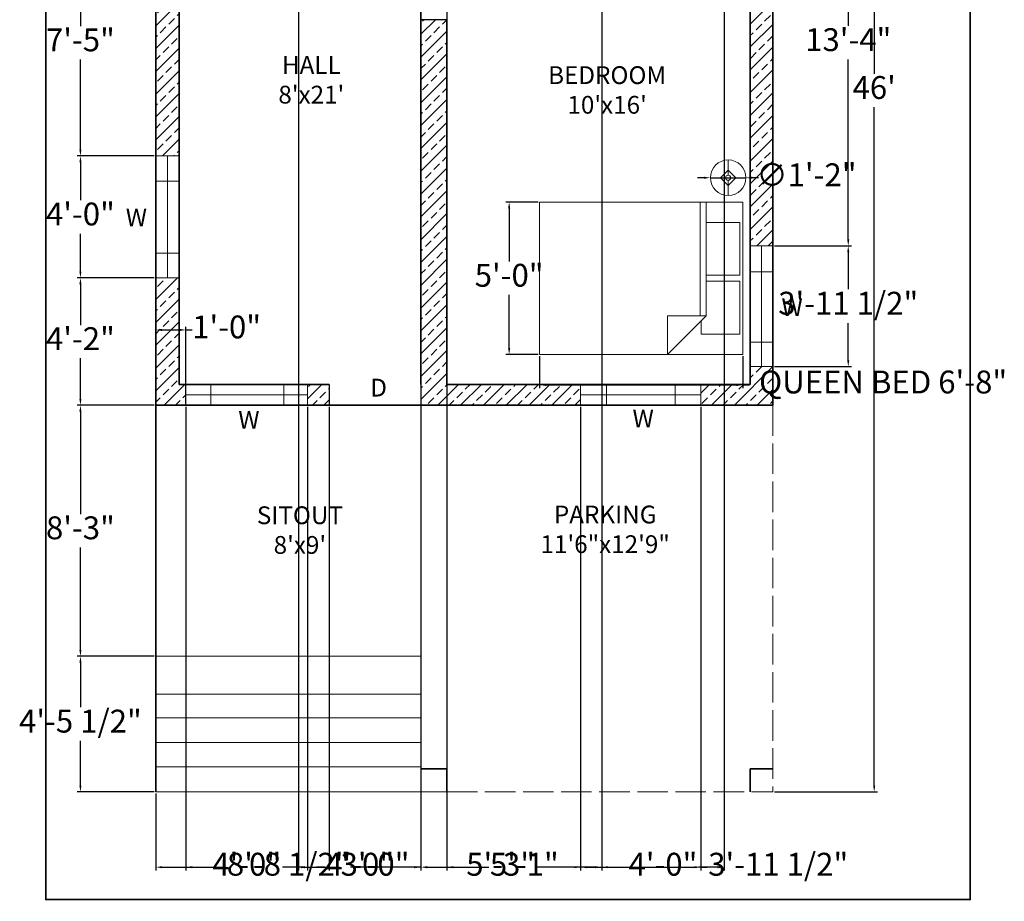
# Model space of a CAD drawing. Units: inches. Extents: x 3686 to 4476, y 4404 to 5066.
# Tile 1 of 2: x 3689 to 4077, y 4404 to 4751. Entities that reach past the tile are written whole.
import ezdxf

# ---------------------------------------------------------------- set-up
doc = ezdxf.new("R2010")
doc.units = ezdxf.units.IN
doc.linetypes.add('ACAD_ISO02W100', pattern=[15, 12, -3])
for name, color, linetype, lineweight in [('A-ANNO-DIMS', 3, 'Continuous', 18), ('A-ANNO-TEXT', 7, 'Continuous', 18), ('A-ANNO-TTLB', 7, 'Continuous', 35), ('A-AREA-IDEN', 7, 'Continuous', 25), ('A-COLS', 7, 'Continuous', 35), ('A-DOOR', 3, 'Continuous', 25), ('A-FLOR-PRKG', 8, 'ACAD_ISO02W100', 18), ('A-FLOR-STRS', 7, 'Continuous', 18), ('A-FURN', 9, 'Continuous', 18), ('A-GLAZ', 4, 'Continuous', 18), ('A-WALL', 7, 'Continuous', 35), ('A-WALL-PATT', 8, 'Continuous', 13)]:
    doc.layers.add(name, color=color, linetype=linetype, lineweight=lineweight)
doc.styles.get("Standard").update_dxf_attribs({"font": 'arial.ttf'})
doc.dimstyles.new('ISO-25', dxfattribs={"dimtxt": 9, "dimasz": 2.5, "dimexe": 1.25, "dimexo": 0.625, "dimgap": 2, "dimtad": 0, "dimtih": 1, "dimtoh": 1, "dimdec": 1, "dimlunit": 4, "dimtxsty": 'Standard', "dimcen": 2.5, "dimadec": 0, "dimazin": 0, "dimtfac": 0.5, "dimtdec": 1, "dimtmove": 0, "dimatfit": 3, "dimfxl": 1, "dimarcsym": 0})

# ---------------------------------------------------------------- blocks, each defined once
blk = doc.blocks.new('*D2')
at = {"layer": 'A-ANNO-DIMS', "color": 0, "lineweight": -2, "transparency": 16777216}
for p, q in [((3986.64, 4999.31), (4027.13, 4999.31)), ((4025.88, 4996.81), (4025.88, 4729.91)), ((4025.88, 4449.81), (4025.88, 4716.72)), ((3986.64, 4447.31), (4027.13, 4447.31))]:
    blk.add_line(p, q, dxfattribs=at)
at = {"layer": 'A-ANNO-DIMS', "color": 0, "transparency": 16777216}
for points in [[(4025.46, 4996.81), (4026.3, 4996.81), (4025.88, 4999.31)], [(4025.46, 4449.81), (4026.3, 4449.81), (4025.88, 4447.31)]]:
    blk.add_solid(points, dxfattribs=at)
at = {"layer": 'Defpoints', "color": 0, "transparency": 16777216}
for p in [(3986.02, 4999.31), (3986.02, 4447.31), (4025.88, 4447.31)]:
    blk.add_point(p, dxfattribs=at)
at = {"layer": 'A-ANNO-DIMS', "color": 0, "transparency": 16777216, "insert": (4025.88, 4723.31), "char_height": 9, "attachment_point": 5}
blk.add_mtext("46'", dxfattribs=at)
blk = doc.blocks.new('Bed - Queen')
for p, q in [((0, -80.00003), (0, 0)), ((0, 0), (59.99999, 0)), ((59.99999, 0), (59.99999, -80.00003)), ((7.99999, -1.2), (28.79998, -1.2)), ((7.99999, -14.4), (7.99999, -1.2)), ((28.79998, -1.2), (28.79998, -14.4)), ((31.19999, -1.2), (51.99999, -1.2)), ((31.19999, -14.4), (31.19999, -1.2)), ((51.99999, -1.2), (51.99999, -16.4)), ((0, -14.4), (44.8, -14.4)), ((59.99999, -29.6), (44.8, -14.4)), ((44.8, -14.4), (44.8, -29.6)), ((44.8, -16.8), (0, -16.8)), ((51.99999, -16.4), (46.79936, -16.4)), ((44.8, -29.6), (59.99999, -29.6)), ((59.99999, -80.00003), (0, -80.00003))]:
    blk.add_line(p, q)
blk = doc.blocks.new('Lamp - Table')
for p, q in [((0, 7), (0, 1)), ((-1, 0), (-7, 0)), ((0, 3), (-3, 0)), ((-3, 0), (0, -3)), ((3, 0), (0, 3)), ((0, -3), (3, 0)), ((1, 0), (7, 0)), ((0, -1), (0, -7))]:
    blk.add_line(p, q)
for radius in [7, 1]:
    blk.add_circle((0, 0), radius)
blk = doc.blocks.new('*D8')
at = {"layer": 'A-ANNO-DIMS', "color": 0, "lineweight": -2, "transparency": 16777216}
for p, q in [((3894.16, 4618.81), (3894.16, 4606.18)), ((3974.16, 4618.81), (3974.16, 4606.18)), ((3896.66, 4607.43), (3971.66, 4607.43)), ((3974.16, 4607.43), (3976.66, 4607.43))]:
    blk.add_line(p, q, dxfattribs=at)
at = {"layer": 'A-ANNO-DIMS', "color": 0, "transparency": 16777216}
for points in [[(3896.66, 4607.85), (3896.66, 4607.02), (3894.16, 4607.43)], [(3971.66, 4607.85), (3971.66, 4607.02), (3974.16, 4607.43)]]:
    blk.add_solid(points, dxfattribs=at)
at = {"layer": 'Defpoints', "color": 0, "transparency": 16777216}
for p in [(3894.16, 4619.43), (3974.16, 4619.43), (3974.16, 4607.43)]:
    blk.add_point(p, dxfattribs=at)
at = {"layer": 'A-ANNO-DIMS', "color": 0, "transparency": 16777216, "insert": (4029.39, 4607.43), "char_height": 9, "attachment_point": 5}
blk.add_mtext('QUEEN BED 6\'-8"', dxfattribs=at)
blk = doc.blocks.new('*D9')
at = {"layer": 'A-ANNO-DIMS', "color": 0, "lineweight": -2, "transparency": 16777216}
for p, q in [((3893.54, 4679.43), (3880.91, 4679.43)), ((3882.16, 4676.93), (3882.16, 4656.03)), ((3882.16, 4621.93), (3882.16, 4642.84)), ((3893.54, 4619.43), (3880.91, 4619.43))]:
    blk.add_line(p, q, dxfattribs=at)
at = {"layer": 'A-ANNO-DIMS', "color": 0, "transparency": 16777216}
for points in [[(3881.75, 4676.93), (3882.58, 4676.93), (3882.16, 4679.43)], [(3881.75, 4621.93), (3882.58, 4621.93), (3882.16, 4619.43)]]:
    blk.add_solid(points, dxfattribs=at)
at = {"layer": 'Defpoints', "color": 0, "transparency": 16777216}
for p in [(3894.16, 4679.43), (3882.16, 4619.43), (3894.16, 4619.43)]:
    blk.add_point(p, dxfattribs=at)
at = {"layer": 'A-ANNO-DIMS', "color": 0, "transparency": 16777216, "insert": (3882.16, 4649.43), "char_height": 9, "attachment_point": 5}
blk.add_mtext('5\'-0"', dxfattribs=at)
blk = doc.blocks.new('*D10')
at = {"layer": 'A-ANNO-DIMS', "color": 0, "lineweight": -2, "transparency": 16777216}
for p, q in [((3742.39, 4599.44), (3712.12, 4599.44)), ((3713.37, 4596.94), (3713.37, 4556.64)), ((3713.37, 4503.15), (3713.37, 4543.45)), ((3742.39, 4500.65), (3712.12, 4500.65))]:
    blk.add_line(p, q, dxfattribs=at)
at = {"layer": 'A-ANNO-DIMS', "color": 0, "transparency": 16777216}
for points in [[(3712.95, 4596.94), (3713.78, 4596.94), (3713.37, 4599.44)], [(3712.95, 4503.15), (3713.78, 4503.15), (3713.37, 4500.65)]]:
    blk.add_solid(points, dxfattribs=at)
at = {"layer": 'Defpoints', "color": 0, "transparency": 16777216}
for p in [(3743.02, 4599.44), (3713.37, 4500.65), (3743.02, 4500.65)]:
    blk.add_point(p, dxfattribs=at)
at = {"layer": 'A-ANNO-DIMS', "color": 0, "transparency": 16777216, "insert": (3713.37, 4550.05), "char_height": 9, "attachment_point": 5}
blk.add_mtext('8\'-3"', dxfattribs=at)
blk = doc.blocks.new('*D11')
at = {"layer": 'A-ANNO-DIMS', "color": 0, "lineweight": -2, "transparency": 16777216}
for p, q in [((3742.39, 4500.65), (3712.12, 4500.65)), ((3713.37, 4498.15), (3713.37, 4480.64)), ((3713.37, 4449.81), (3713.37, 4467.33)), ((3742.39, 4447.31), (3712.12, 4447.31))]:
    blk.add_line(p, q, dxfattribs=at)
at = {"layer": 'A-ANNO-DIMS', "color": 0, "transparency": 16777216}
for points in [[(3712.95, 4498.15), (3713.78, 4498.15), (3713.37, 4500.65)], [(3712.95, 4449.81), (3713.78, 4449.81), (3713.37, 4447.31)]]:
    blk.add_solid(points, dxfattribs=at)
at = {"layer": 'Defpoints', "color": 0, "transparency": 16777216}
for p in [(3743.02, 4500.65), (3713.37, 4447.31), (3743.02, 4447.31)]:
    blk.add_point(p, dxfattribs=at)
at = {"layer": 'A-ANNO-DIMS', "color": 0, "transparency": 16777216, "insert": (3713.37, 4473.98), "char_height": 9, "attachment_point": 5}
blk.add_mtext('4\'-5 1/2"', dxfattribs=at)
blk = doc.blocks.new('*D12')
at = {"layer": 'A-ANNO-DIMS', "color": 0, "lineweight": -2, "transparency": 16777216}
for p, q in [((3743.02, 4446.69), (3743.02, 4416.41)), ((3847.39, 4446.69), (3847.39, 4416.41)), ((3745.52, 4417.66), (3770.75, 4417.66)), ((3844.89, 4417.66), (3819.66, 4417.66))]:
    blk.add_line(p, q, dxfattribs=at)
at = {"layer": 'A-ANNO-DIMS', "color": 0, "transparency": 16777216}
for points in [[(3745.52, 4418.08), (3745.52, 4417.25), (3743.02, 4417.66)], [(3844.89, 4418.08), (3844.89, 4417.25), (3847.39, 4417.66)]]:
    blk.add_solid(points, dxfattribs=at)
at = {"layer": 'Defpoints', "color": 0, "transparency": 16777216}
for p in [(3743.02, 4447.31), (3847.39, 4447.31), (3847.39, 4417.66)]:
    blk.add_point(p, dxfattribs=at)
at = {"layer": 'A-ANNO-DIMS', "color": 0, "transparency": 16777216, "insert": (3795.2, 4417.66), "char_height": 9, "attachment_point": 5}
blk.add_mtext('8\'-8 1/2"', dxfattribs=at)
blk = doc.blocks.new('*D14')
at = {"layer": 'A-ANNO-DIMS', "color": 0, "lineweight": -2, "transparency": 16777216}
for p, q in [((3857.64, 4987.97), (3857.64, 4416.41)), ((3918.61, 4987.97), (3918.61, 4416.41)), ((3860.14, 4417.66), (3874.16, 4417.66)), ((3916.11, 4417.66), (3902.09, 4417.66))]:
    blk.add_line(p, q, dxfattribs=at)
at = {"layer": 'A-ANNO-DIMS', "color": 0, "transparency": 16777216}
for points in [[(3860.14, 4418.08), (3860.14, 4417.25), (3857.64, 4417.66)], [(3916.11, 4418.08), (3916.11, 4417.25), (3918.61, 4417.66)]]:
    blk.add_solid(points, dxfattribs=at)
at = {"layer": 'Defpoints', "color": 0, "transparency": 16777216}
for p in [(3857.64, 4988.59), (3918.61, 4988.59), (3918.61, 4417.66)]:
    blk.add_point(p, dxfattribs=at)
at = {"layer": 'A-ANNO-DIMS', "color": 0, "transparency": 16777216, "insert": (3888.13, 4417.66), "char_height": 9, "attachment_point": 5}
blk.add_mtext('5\'-1"', dxfattribs=at)
blk = doc.blocks.new('*D15')
at = {"layer": 'A-ANNO-DIMS', "color": 0, "lineweight": -2, "transparency": 16777216}
for p, q in [((3918.61, 4987.97), (3918.61, 4416.41)), ((3966.81, 4987.97), (3966.81, 4416.41)), ((3921.11, 4417.66), (3928.57, 4417.66)), ((3964.31, 4417.66), (3956.85, 4417.66))]:
    blk.add_line(p, q, dxfattribs=at)
at = {"layer": 'A-ANNO-DIMS', "color": 0, "transparency": 16777216}
for points in [[(3921.11, 4418.08), (3921.11, 4417.25), (3918.61, 4417.66)], [(3964.31, 4418.08), (3964.31, 4417.25), (3966.81, 4417.66)]]:
    blk.add_solid(points, dxfattribs=at)
at = {"layer": 'Defpoints', "color": 0, "transparency": 16777216}
for p in [(3918.61, 4988.59), (3966.81, 4988.59), (3966.81, 4417.66)]:
    blk.add_point(p, dxfattribs=at)
at = {"layer": 'A-ANNO-DIMS', "color": 0, "transparency": 16777216, "insert": (3942.71, 4417.66), "char_height": 9, "attachment_point": 5}
blk.add_mtext('4\'-0"', dxfattribs=at)
blk = doc.blocks.new('*D20')
at = {"layer": 'A-ANNO-DIMS', "color": 0, "lineweight": -2, "transparency": 16777216}
for p, q in [((3986.64, 4822.12), (4016.92, 4822.12)), ((4015.67, 4819.62), (4015.67, 4748.74)), ((4015.67, 4664.68), (4015.67, 4735.55)), ((3986.64, 4662.18), (4016.92, 4662.18))]:
    blk.add_line(p, q, dxfattribs=at)
at = {"layer": 'A-ANNO-DIMS', "color": 0, "transparency": 16777216}
for points in [[(4015.25, 4819.62), (4016.08, 4819.62), (4015.67, 4822.12)], [(4015.25, 4664.68), (4016.08, 4664.68), (4015.67, 4662.18)]]:
    blk.add_solid(points, dxfattribs=at)
at = {"layer": 'Defpoints', "color": 0, "transparency": 16777216}
for p in [(3986.02, 4822.12), (3986.02, 4662.18), (4015.67, 4662.18)]:
    blk.add_point(p, dxfattribs=at)
at = {"layer": 'A-ANNO-DIMS', "color": 0, "transparency": 16777216, "insert": (4015.67, 4742.15), "char_height": 9, "attachment_point": 5}
blk.add_mtext('13\'-4"', dxfattribs=at)
blk = doc.blocks.new('*D21')
at = {"layer": 'A-ANNO-DIMS', "color": 0, "lineweight": -2, "transparency": 16777216}
for p, q in [((3986.64, 4662.18), (4016.92, 4662.18)), ((4015.67, 4659.68), (4015.67, 4645.09)), ((4015.67, 4617.19), (4015.67, 4631.78)), ((3986.64, 4614.69), (4016.92, 4614.69))]:
    blk.add_line(p, q, dxfattribs=at)
at = {"layer": 'A-ANNO-DIMS', "color": 0, "transparency": 16777216}
for points in [[(4015.25, 4659.68), (4016.08, 4659.68), (4015.67, 4662.18)], [(4015.25, 4617.19), (4016.08, 4617.19), (4015.67, 4614.69)]]:
    blk.add_solid(points, dxfattribs=at)
at = {"layer": 'Defpoints', "color": 0, "transparency": 16777216}
for p in [(3986.02, 4662.18), (3986.02, 4614.69), (4015.67, 4614.69)]:
    blk.add_point(p, dxfattribs=at)
at = {"layer": 'A-ANNO-DIMS', "color": 0, "transparency": 16777216, "insert": (4015.67, 4638.43), "char_height": 9, "attachment_point": 5}
blk.add_mtext('3\'-11 1/2"', dxfattribs=at)
blk = doc.blocks.new('*D25')
at = {"layer": 'A-ANNO-DIMS', "color": 0, "lineweight": -2, "transparency": 16777216}
for p, q in [((3742.39, 4786.58), (3712.12, 4786.58)), ((3713.37, 4784.08), (3713.37, 4748.64)), ((3713.37, 4700.05), (3713.37, 4735.49)), ((3742.39, 4697.55), (3712.12, 4697.55))]:
    blk.add_line(p, q, dxfattribs=at)
at = {"layer": 'A-ANNO-DIMS', "color": 0, "transparency": 16777216}
for points in [[(3712.95, 4784.08), (3713.78, 4784.08), (3713.37, 4786.58)], [(3712.95, 4700.05), (3713.78, 4700.05), (3713.37, 4697.55)]]:
    blk.add_solid(points, dxfattribs=at)
at = {"layer": 'Defpoints', "color": 0, "transparency": 16777216}
for p in [(3743.02, 4786.58), (3713.37, 4697.55), (3743.02, 4697.55)]:
    blk.add_point(p, dxfattribs=at)
at = {"layer": 'A-ANNO-DIMS', "color": 0, "transparency": 16777216, "insert": (3713.37, 4742.07), "char_height": 9, "attachment_point": 5}
blk.add_mtext('7\'-5"', dxfattribs=at)
blk = doc.blocks.new('*D26')
at = {"layer": 'A-ANNO-DIMS', "color": 0, "lineweight": -2, "transparency": 16777216}
for p, q in [((3742.39, 4697.55), (3712.12, 4697.55)), ((3713.37, 4695.05), (3713.37, 4680.14)), ((3713.37, 4652.05), (3713.37, 4666.95)), ((3742.39, 4649.55), (3712.12, 4649.55))]:
    blk.add_line(p, q, dxfattribs=at)
at = {"layer": 'A-ANNO-DIMS', "color": 0, "transparency": 16777216}
for points in [[(3712.95, 4695.05), (3713.78, 4695.05), (3713.37, 4697.55)], [(3712.95, 4652.05), (3713.78, 4652.05), (3713.37, 4649.55)]]:
    blk.add_solid(points, dxfattribs=at)
at = {"layer": 'Defpoints', "color": 0, "transparency": 16777216}
for p in [(3743.02, 4697.55), (3713.37, 4649.55), (3743.02, 4649.55)]:
    blk.add_point(p, dxfattribs=at)
at = {"layer": 'A-ANNO-DIMS', "color": 0, "transparency": 16777216, "insert": (3713.37, 4673.55), "char_height": 9, "attachment_point": 5}
blk.add_mtext('4\'-0"', dxfattribs=at)
blk = doc.blocks.new('*D27')
at = {"layer": 'A-ANNO-DIMS', "color": 0, "lineweight": -2, "transparency": 16777216}
for p, q in [((3742.39, 4649.55), (3712.12, 4649.55)), ((3713.37, 4647.05), (3713.37, 4631.01)), ((3713.37, 4601.94), (3713.37, 4617.98)), ((3742.39, 4599.44), (3712.12, 4599.44))]:
    blk.add_line(p, q, dxfattribs=at)
at = {"layer": 'A-ANNO-DIMS', "color": 0, "transparency": 16777216}
for points in [[(3712.95, 4647.05), (3713.78, 4647.05), (3713.37, 4649.55)], [(3712.95, 4601.94), (3713.78, 4601.94), (3713.37, 4599.44)]]:
    blk.add_solid(points, dxfattribs=at)
at = {"layer": 'Defpoints', "color": 0, "transparency": 16777216}
for p in [(3743.02, 4649.55), (3713.37, 4599.44), (3743.02, 4599.44)]:
    blk.add_point(p, dxfattribs=at)
at = {"layer": 'A-ANNO-DIMS', "color": 0, "transparency": 16777216, "insert": (3713.37, 4624.49), "char_height": 9, "attachment_point": 5}
blk.add_mtext('4\'-2"', dxfattribs=at)
blk = doc.blocks.new('*D28')
at = {"layer": 'A-ANNO-DIMS', "color": 0, "lineweight": -2, "transparency": 16777216}
for p, q in [((3743.02, 4600.06), (3743.02, 4630.34)), ((3745.52, 4629.09), (3752.38, 4629.09)), ((3754.88, 4600.06), (3754.88, 4630.34)), ((3754.88, 4629.09), (3757.38, 4629.09))]:
    blk.add_line(p, q, dxfattribs=at)
at = {"layer": 'A-ANNO-DIMS', "color": 0, "transparency": 16777216}
for points in [[(3745.52, 4629.51), (3745.52, 4628.67), (3743.02, 4629.09)], [(3752.38, 4629.51), (3752.38, 4628.67), (3754.88, 4629.09)]]:
    blk.add_solid(points, dxfattribs=at)
at = {"layer": 'Defpoints', "color": 0, "transparency": 16777216}
for p in [(3754.88, 4629.09), (3743.02, 4599.44), (3754.88, 4599.44)]:
    blk.add_point(p, dxfattribs=at)
at = {"layer": 'A-ANNO-DIMS', "color": 0, "transparency": 16777216, "insert": (3770.92, 4629.09), "char_height": 9, "attachment_point": 5}
blk.add_mtext('1\'-0"', dxfattribs=at)
blk = doc.blocks.new('*D29')
at = {"layer": 'A-ANNO-DIMS', "color": 0, "lineweight": -2, "transparency": 16777216}
for p, q in [((3754.88, 4598.81), (3754.88, 4416.41)), ((3802.75, 4598.81), (3802.75, 4416.41)), ((3757.38, 4417.66), (3764.67, 4417.66)), ((3800.25, 4417.66), (3792.96, 4417.66))]:
    blk.add_line(p, q, dxfattribs=at)
at = {"layer": 'A-ANNO-DIMS', "color": 0, "transparency": 16777216}
for points in [[(3757.38, 4418.08), (3757.38, 4417.25), (3754.88, 4417.66)], [(3800.25, 4418.08), (3800.25, 4417.25), (3802.75, 4417.66)]]:
    blk.add_solid(points, dxfattribs=at)
at = {"layer": 'Defpoints', "color": 0, "transparency": 16777216}
for p in [(3754.88, 4599.44), (3802.75, 4599.44), (3802.75, 4417.66)]:
    blk.add_point(p, dxfattribs=at)
at = {"layer": 'A-ANNO-DIMS', "color": 0, "transparency": 16777216, "insert": (3778.82, 4417.66), "char_height": 9, "attachment_point": 5}
blk.add_mtext('4\'-0"', dxfattribs=at)
blk = doc.blocks.new('*D30')
at = {"layer": 'A-ANNO-DIMS', "color": 0, "lineweight": -2, "transparency": 16777216}
for p, q in [((3811.33, 4598.81), (3811.33, 4416.41)), ((3847.39, 4598.81), (3847.39, 4416.41)), ((3808.83, 4417.66), (3806.33, 4417.66)), ((3811.33, 4417.66), (3815.4, 4417.66)), ((3847.39, 4417.66), (3843.32, 4417.66)), ((3849.89, 4417.66), (3852.39, 4417.66))]:
    blk.add_line(p, q, dxfattribs=at)
at = {"layer": 'A-ANNO-DIMS', "color": 0, "transparency": 16777216}
for points in [[(3808.83, 4418.08), (3808.83, 4417.25), (3811.33, 4417.66)], [(3849.89, 4418.08), (3849.89, 4417.25), (3847.39, 4417.66)]]:
    blk.add_solid(points, dxfattribs=at)
at = {"layer": 'Defpoints', "color": 0, "transparency": 16777216}
for p in [(3811.33, 4599.44), (3847.39, 4599.44), (3847.39, 4417.66)]:
    blk.add_point(p, dxfattribs=at)
at = {"layer": 'A-ANNO-DIMS', "color": 0, "transparency": 16777216, "insert": (3829.36, 4417.66), "char_height": 9, "attachment_point": 5}
blk.add_mtext('3\'-0"', dxfattribs=at)
blk = doc.blocks.new('*D31')
at = {"layer": 'A-ANNO-DIMS', "color": 0, "lineweight": -2, "transparency": 16777216}
for p, q in [((3847.39, 4598.81), (3847.39, 4416.41)), ((3910.28, 4598.81), (3910.28, 4416.41)), ((3849.89, 4417.66), (3864.87, 4417.66)), ((3907.78, 4417.66), (3892.8, 4417.66))]:
    blk.add_line(p, q, dxfattribs=at)
at = {"layer": 'A-ANNO-DIMS', "color": 0, "transparency": 16777216}
for points in [[(3849.89, 4418.08), (3849.89, 4417.25), (3847.39, 4417.66)], [(3907.78, 4418.08), (3907.78, 4417.25), (3910.28, 4417.66)]]:
    blk.add_solid(points, dxfattribs=at)
at = {"layer": 'Defpoints', "color": 0, "transparency": 16777216}
for p in [(3847.39, 4599.44), (3910.28, 4599.44), (3910.28, 4417.66)]:
    blk.add_point(p, dxfattribs=at)
at = {"layer": 'A-ANNO-DIMS', "color": 0, "transparency": 16777216, "insert": (3878.83, 4417.66), "char_height": 9, "attachment_point": 5}
blk.add_mtext('5\'-3"', dxfattribs=at)
blk = doc.blocks.new('*D32')
at = {"layer": 'A-ANNO-DIMS', "color": 0, "lineweight": -2, "transparency": 16777216}
for p, q in [((3910.28, 4598.81), (3910.28, 4416.41)), ((3957.66, 4598.81), (3957.66, 4416.41)), ((3912.78, 4417.66), (3955.16, 4417.66)), ((3957.66, 4417.66), (3960.16, 4417.66))]:
    blk.add_line(p, q, dxfattribs=at)
at = {"layer": 'A-ANNO-DIMS', "color": 0, "transparency": 16777216}
for points in [[(3912.78, 4418.08), (3912.78, 4417.25), (3910.28, 4417.66)], [(3955.16, 4418.08), (3955.16, 4417.25), (3957.66, 4417.66)]]:
    blk.add_solid(points, dxfattribs=at)
at = {"layer": 'Defpoints', "color": 0, "transparency": 16777216}
for p in [(3910.28, 4599.44), (3957.66, 4599.44), (3957.66, 4417.66)]:
    blk.add_point(p, dxfattribs=at)
at = {"layer": 'A-ANNO-DIMS', "color": 0, "transparency": 16777216, "insert": (3988.1, 4417.66), "char_height": 9, "attachment_point": 5}
blk.add_mtext('3\'-11 1/2"', dxfattribs=at)
blk = doc.blocks.new('*D35')
at = {"layer": 'A-ANNO-DIMS', "color": 0, "lineweight": -2, "transparency": 16777216}
for p, q in [((3799.26, 4857.46), (3799.26, 4416.41)), ((3847.39, 4857.46), (3847.39, 4416.41)), ((3801.76, 4417.66), (3809.18, 4417.66)), ((3844.89, 4417.66), (3837.47, 4417.66))]:
    blk.add_line(p, q, dxfattribs=at)
at = {"layer": 'A-ANNO-DIMS', "color": 0, "transparency": 16777216}
for points in [[(3801.76, 4418.08), (3801.76, 4417.25), (3799.26, 4417.66)], [(3844.89, 4418.08), (3844.89, 4417.25), (3847.39, 4417.66)]]:
    blk.add_solid(points, dxfattribs=at)
at = {"layer": 'Defpoints', "color": 0, "transparency": 16777216}
for p in [(3799.26, 4858.09), (3847.39, 4858.09), (3847.39, 4417.66)]:
    blk.add_point(p, dxfattribs=at)
at = {"layer": 'A-ANNO-DIMS', "color": 0, "transparency": 16777216, "insert": (3823.32, 4417.66), "char_height": 9, "attachment_point": 5}
blk.add_mtext('4\'-0"', dxfattribs=at)
blk = doc.blocks.new('*D37')
at = {"layer": 'A-ANNO-DIMS', "color": 0, "lineweight": -2, "transparency": 16777216}
for p, q in [((3958.87, 4688.98), (3956.37, 4688.98)), ((3961.37, 4688.98), (3975.37, 4688.98)), ((3980.37, 4688.98), (3977.87, 4688.98))]:
    blk.add_line(p, q, dxfattribs=at)
at = {"layer": 'A-ANNO-DIMS', "color": 0, "transparency": 16777216}
for points in [[(3958.87, 4689.39), (3958.87, 4688.56), (3961.37, 4688.98)], [(3977.87, 4689.39), (3977.87, 4688.56), (3975.37, 4688.98)]]:
    blk.add_solid(points, dxfattribs=at)
at = {"layer": 'Defpoints', "color": 0, "transparency": 16777216}
for p in [(3961.37, 4688.98), (3975.37, 4688.98)]:
    blk.add_point(p, dxfattribs=at)
at = {"layer": 'A-ANNO-DIMS', "color": 0, "transparency": 16777216, "insert": (3999.23, 4688.98), "char_height": 9, "attachment_point": 5}
blk.add_mtext('∅1\'-2"', dxfattribs=at)

msp = doc.modelspace()

# ---------------------------------------------------------------- hatches: boundary and pattern name
at = {"layer": 'A-WALL-PATT'}
h = msp.add_hatch(dxfattribs=at)
h.set_pattern_fill('ANSI33', color=256)
h.paths.add_polyline_path([(3810.64, 4999.31), (3743.02, 4999.31), (3743.02, 4952.43), (3752.2, 4952.43), (3752.2, 4988.59), (3810.64, 4988.59)])
h.paths.add_polyline_path([(3918.61, 4999.31), (3847.39, 4999.31), (3847.39, 4988.59), (3847.39, 4913.66), (3857.64, 4913.66), (3857.64, 4988.59), (3918.61, 4988.59)])
h.paths.add_polyline_path([(3986.02, 4999.31), (3966.81, 4999.31), (3966.81, 4988.59), (3977.11, 4988.59), (3977.11, 4952.21), (3986.02, 4952.21)])
h.paths.add_polyline_path([(3986.02, 4904.23), (3977.11, 4904.23), (3977.11, 4868.69), (3857.64, 4868.69), (3847.39, 4868.69), (3847.39, 4858.09), (3847.39, 4799.25), (3857.64, 4799.25), (3949.83, 4799.25), (3949.83, 4804.86), (3857.64, 4804.86), (3857.64, 4862.27), (3977.11, 4862.27), (3977.11, 4845.08), (3986.02, 4845.08)])
h.paths.add_polyline_path([(3986.02, 4822.12), (3977.11, 4822.12), (3977.11, 4662.18), (3986.02, 4662.18)])
h.paths.add_polyline_path([(3857.64, 4751.17), (3847.39, 4751.17), (3847.39, 4607.62), (3847.39, 4599.44), (3910.28, 4599.44), (3910.28, 4607.62), (3857.64, 4607.62)])
h.paths.add_polyline_path([(3986.02, 4614.69), (3977.11, 4614.69), (3977.11, 4607.62), (3957.66, 4607.62), (3957.66, 4599.44), (3986.02, 4599.44)])
h.paths.add_polyline_path([(3811.33, 4607.62), (3802.75, 4607.62), (3802.75, 4599.44), (3811.33, 4599.44)])
h.paths.add_polyline_path([(3752.2, 4649.55), (3743.02, 4649.55), (3743.02, 4599.44), (3754.88, 4599.44), (3754.88, 4607.62), (3752.2, 4607.62)])
h.paths.add_polyline_path([(3752.2, 4786.58), (3743.02, 4786.58), (3743.02, 4697.55), (3752.2, 4697.55)])
h.paths.add_polyline_path([(3799.26, 4868.69), (3752.2, 4868.69), (3752.2, 4904.87), (3743.02, 4904.87), (3743.02, 4835.05), (3752.2, 4835.05), (3752.2, 4858.09), (3799.26, 4858.09)])

# ---------------------------------------------------------------- linework, layer by layer
at = {"layer": 'A-ANNO-TTLB'}
msp.add_lwpolyline([(3699.7, 5065.96), (4063.67, 5065.96), (4063.67, 4404.9), (3699.7, 4404.9)], close=True, dxfattribs=at)
at = {"layer": 'A-COLS'}
for p, q in [((3857.64, 4456.31), (3847.39, 4456.31)), ((3857.64, 4456.31), (3857.64, 4447.31)), ((3857.64, 4447.31), (3857.64, 4456.31)), ((3977.11, 4456.31), (3986.02, 4456.31)), ((3977.11, 4456.31), (3977.11, 4447.31))]:
    msp.add_line(p, q, dxfattribs=at)
at = {"layer": 'A-DOOR'}
for p, q in [((3857.64, 4751.17), (3847.39, 4751.17)), ((3811.33, 4607.62), (3811.33, 4599.44)), ((3847.39, 4607.62), (3847.39, 4599.44))]:
    msp.add_line(p, q, dxfattribs=at)
at = {"layer": 'A-FLOR-PRKG'}
for p, q in [((3847.39, 4447.31), (3847.39, 4599.44)), ((3986.02, 4599.44), (3986.02, 4447.31)), ((3857.64, 4447.31), (3986.02, 4447.31))]:
    msp.add_line(p, q, dxfattribs=at)
at = {"layer": 'A-FLOR-STRS'}
for p, q in [((3743.02, 4500.65), (3847.39, 4500.65)), ((3743.02, 4485.76), (3847.39, 4485.76)), ((3743.02, 4476.38), (3847.39, 4476.38)), ((3743.02, 4466.7), (3847.39, 4466.7)), ((3743.02, 4457.18), (3847.39, 4457.18)), ((3743.02, 4447.31), (3857.64, 4447.31)), ((3743.02, 4447.31), (3847.39, 4447.31))]:
    msp.add_line(p, q, dxfattribs=at)
at = {"layer": 'A-GLAZ'}
for p, q in [((3743.02, 4697.55), (3752.2, 4697.55)), ((3747.61, 4697.55), (3747.61, 4649.55)), ((3743.02, 4687.65), (3752.2, 4687.65)), ((3977.11, 4662.18), (3986.02, 4662.18)), ((3981.56, 4662.18), (3981.56, 4614.69)), ((3743.02, 4659.36), (3752.2, 4659.36)), ((3977.11, 4652.01), (3986.02, 4652.01)), ((3743.02, 4649.55), (3752.2, 4649.55)), ((3977.11, 4624.28), (3986.02, 4624.28)), ((3977.11, 4614.69), (3986.02, 4614.69)), ((3754.88, 4607.62), (3754.88, 4599.44)), ((3764.67, 4607.62), (3764.67, 4599.44)), ((3793.42, 4607.62), (3793.42, 4599.44)), ((3802.75, 4607.62), (3802.75, 4599.44)), ((3910.28, 4607.62), (3910.28, 4599.44)), ((3920.55, 4607.62), (3920.55, 4599.44)), ((3947.57, 4607.62), (3947.57, 4599.44)), ((3957.66, 4607.62), (3957.66, 4599.44)), ((3754.88, 4603.53), (3802.75, 4603.53)), ((3957.66, 4603.53), (3910.28, 4603.53))]:
    msp.add_line(p, q, dxfattribs=at)
at = {"layer": 'A-WALL'}
for p, q in [((3743.02, 4447.31), (3743.02, 4999.31)), ((3986.02, 4599.44), (3986.02, 4999.31)), ((3977.11, 4862.27), (3977.11, 4607.62)), ((3752.2, 4607.62), (3752.2, 4858.09)), ((3847.39, 4607.62), (3847.39, 4858.09)), ((3857.64, 4607.62), (3857.64, 4751.17)), ((3811.33, 4607.62), (3752.2, 4607.62)), ((3857.64, 4607.62), (3977.11, 4607.62)), ((3847.39, 4599.44), (3743.02, 4599.44)), ((3847.39, 4599.44), (3986.02, 4599.44))]:
    msp.add_line(p, q, dxfattribs=at)

# ---------------------------------------------------------------- block references
at = {"layer": 'A-FURN'}
msp.add_blockref('Lamp - Table', (3968.37, 4688.98), dxfattribs=at)
at = {"layer": 'A-FURN', "rotation": 270}
msp.add_blockref('Bed - Queen', (3974.16, 4679.43), dxfattribs=at)

# ---------------------------------------------------------------- texts
at = {"layer": 'A-ANNO-TEXT', "char_height": 7, "attachment_point": 1}
for s, insert in [('\\pxqc;{\\fArial|b1|i0|c0|p34;W}', (3724.65, 4676.87)), ('\\pxqc;{\\fArial|b1|i0|c0|p34;W}', (3982.81, 4641.51)), ('\\pxqc;{\\fArial|b1|i0|c0|p34;D}', (3820.03, 4609.88)), ('\\pxqc;{\\fArial|b1|i0|c0|p34;W}', (3924.17, 4597.7)), ('\\pxqc;{\\fArial|b1|i0|c0|p34;W}', (3768.95, 4597.22))]:
    msp.add_mtext_dynamic_manual_height_columns(s, width=21.499, gutter_width=12.5, heights=[0], dxfattribs=dict(at, insert=insert))
at = {"layer": 'A-AREA-IDEN', "char_height": 7, "attachment_point": 1}
for s, width, insert in [("\\pxqc;{\\fArial|b1|i0|c0|p34;HALL\\P8'x21'}", 72.6922, (3767.93, 4736.85)), ("\\pxqc;{\\fArial|b1|i0|c0|p34;BEDROOM\\P10'x16'}", 87.3509, (3877.06, 4732.85)), ("\\pxqc;{\\fArial|b1|i0|c0|p34;SITOUT\\P8'x9'}", 57.1608, (3771.19, 4559.65)), ('\\pxqc;{\\fArial|b1|i0|c0|p34;PARKING\\P11\'6"x12\'9"}', 103.792, (3868.07, 4559.95))]:
    msp.add_mtext_dynamic_manual_height_columns(s, width=width, gutter_width=12.5, heights=[0], dxfattribs=dict(at, insert=insert))

# ---------------------------------------------------------------- dimensions: what is measured, and where the dimension line sits
at = {"layer": 'A-ANNO-DIMS'}
for base, p1, p2, angle, override, picture, middle in [((4025.88, 4447.31), (3986.02, 4999.31), (3986.02, 4447.31), 90, {"dimclrd": 0, "dimclre": 0, "dimclrt": 0}, '*D2', (4025.88, 4723.31)), ((4015.67, 4662.18), (3986.02, 4822.12), (3986.02, 4662.18), 90, {"dimdec": 1, "dimlfac": 1, "dimrnd": 0, "dimzin": 1, "dimdsep": 46, "dimlunit": 4, "dimfrac": 2}, '*D20', (4015.67, 4742.15)), ((3713.37, 4697.55), (3743.02, 4786.58), (3743.02, 4697.55), 90, {"dimdec": 1, "dimlfac": 1, "dimrnd": 0, "dimzin": 1, "dimdsep": 46, "dimlunit": 4, "dimfrac": 2}, '*D25', (3713.37, 4742.07)), ((3713.37, 4649.55), (3743.02, 4697.55), (3743.02, 4649.55), 90, {"dimdec": 1, "dimlfac": 1, "dimrnd": 0, "dimzin": 1, "dimdsep": 46, "dimlunit": 4, "dimfrac": 2}, '*D26', (3713.37, 4673.55)), ((3882.16, 4619.43), (3894.16, 4679.43), (3894.16, 4619.43), 270, {"dimdec": 1, "dimlfac": 1, "dimrnd": 0, "dimzin": 1, "dimdsep": 46, "dimlunit": 4, "dimfrac": 2}, '*D9', (3882.16, 4649.43)), ((4015.67, 4614.69), (3986.02, 4662.18), (3986.02, 4614.69), 90, {"dimdec": 1, "dimlfac": 1, "dimrnd": 0, "dimzin": 1, "dimdsep": 46, "dimlunit": 4, "dimfrac": 2}, '*D21', (4015.67, 4638.43)), ((3713.37, 4599.44), (3743.02, 4649.55), (3743.02, 4599.44), 90, {"dimdec": 1, "dimlfac": 1, "dimrnd": 0, "dimzin": 1, "dimdsep": 46, "dimlunit": 4, "dimfrac": 2}, '*D27', (3713.37, 4624.49)), ((3713.37, 4500.65), (3743.02, 4599.44), (3743.02, 4500.65), 90, {"dimdec": 1, "dimlfac": 1, "dimrnd": 0, "dimzin": 1, "dimdsep": 46, "dimlunit": 4, "dimfrac": 2}, '*D10', (3713.37, 4550.05)), ((3713.37, 4447.31), (3743.02, 4500.65), (3743.02, 4447.31), 90, {"dimdec": 1, "dimlfac": 1, "dimrnd": 0, "dimzin": 1, "dimdsep": 46, "dimlunit": 4, "dimfrac": 2}, '*D11', (3713.37, 4473.98))]:
    dim = msp.add_linear_dim(base=base, p1=p1, p2=p2, angle=angle, dimstyle='ISO-25', override=override, dxfattribs=at)
    dim.commit()
    dim.dimension.update_dxf_attribs({"geometry": picture, "text_midpoint": middle})
for base, p1, p2, picture, middle in [((3918.61, 4417.66), (3857.64, 4988.59), (3918.61, 4988.59), '*D14', (3888.13, 4417.66)), ((3966.81, 4417.66), (3918.61, 4988.59), (3966.81, 4988.59), '*D15', (3942.71, 4417.66)), ((3847.39, 4417.66), (3799.26, 4858.09), (3847.39, 4858.09), '*D35', (3823.32, 4417.66)), ((3754.88, 4629.09), (3743.02, 4599.44), (3754.88, 4599.44), '*D28', (3770.92, 4629.09)), ((3802.75, 4417.66), (3754.88, 4599.44), (3802.75, 4599.44), '*D29', (3778.82, 4417.66)), ((3847.39, 4417.66), (3811.33, 4599.44), (3847.39, 4599.44), '*D30', (3829.36, 4417.66)), ((3910.28, 4417.66), (3847.39, 4599.44), (3910.28, 4599.44), '*D31', (3878.83, 4417.66)), ((3957.66, 4417.66), (3910.28, 4599.44), (3957.66, 4599.44), '*D32', (3988.1, 4417.66)), ((3847.39, 4417.66), (3743.02, 4447.31), (3847.39, 4447.31), '*D12', (3795.2, 4417.66))]:
    dim = msp.add_linear_dim(base=base, p1=p1, p2=p2, dimstyle='ISO-25', override={"dimdec": 1, "dimlfac": 1, "dimrnd": 0, "dimzin": 1, "dimdsep": 46, "dimlunit": 4, "dimfrac": 2}, dxfattribs=at)
    dim.commit()
    dim.dimension.update_dxf_attribs({"geometry": picture, "text_midpoint": middle})
dim = msp.add_diameter_dim_2p(p1=(3961.37, 4688.98), p2=(3975.37, 4688.98), dimstyle='ISO-25', override={"dimdec": 1, "dimlfac": 1, "dimrnd": 0, "dimzin": 1, "dimdsep": 46, "dimlunit": 4, "dimfrac": 2}, dxfattribs=at)
dim.commit()
dim.dimension.update_dxf_attribs({"geometry": '*D37', "text_midpoint": (3980.37, 4688.98)})
dim = msp.add_linear_dim(base=(3974.16, 4607.43), p1=(3894.16, 4619.43), p2=(3974.16, 4619.43), text='QUEEN BED <>', dimstyle='ISO-25', override={"dimdec": 1, "dimlfac": 1, "dimrnd": 0, "dimzin": 1, "dimdsep": 46, "dimlunit": 4, "dimfrac": 2}, dxfattribs=at)
dim.commit()
dim.dimension.update_dxf_attribs({"geometry": '*D8', "text_midpoint": (4029.39, 4607.43)})

doc.saveas('drawing.dxf')
